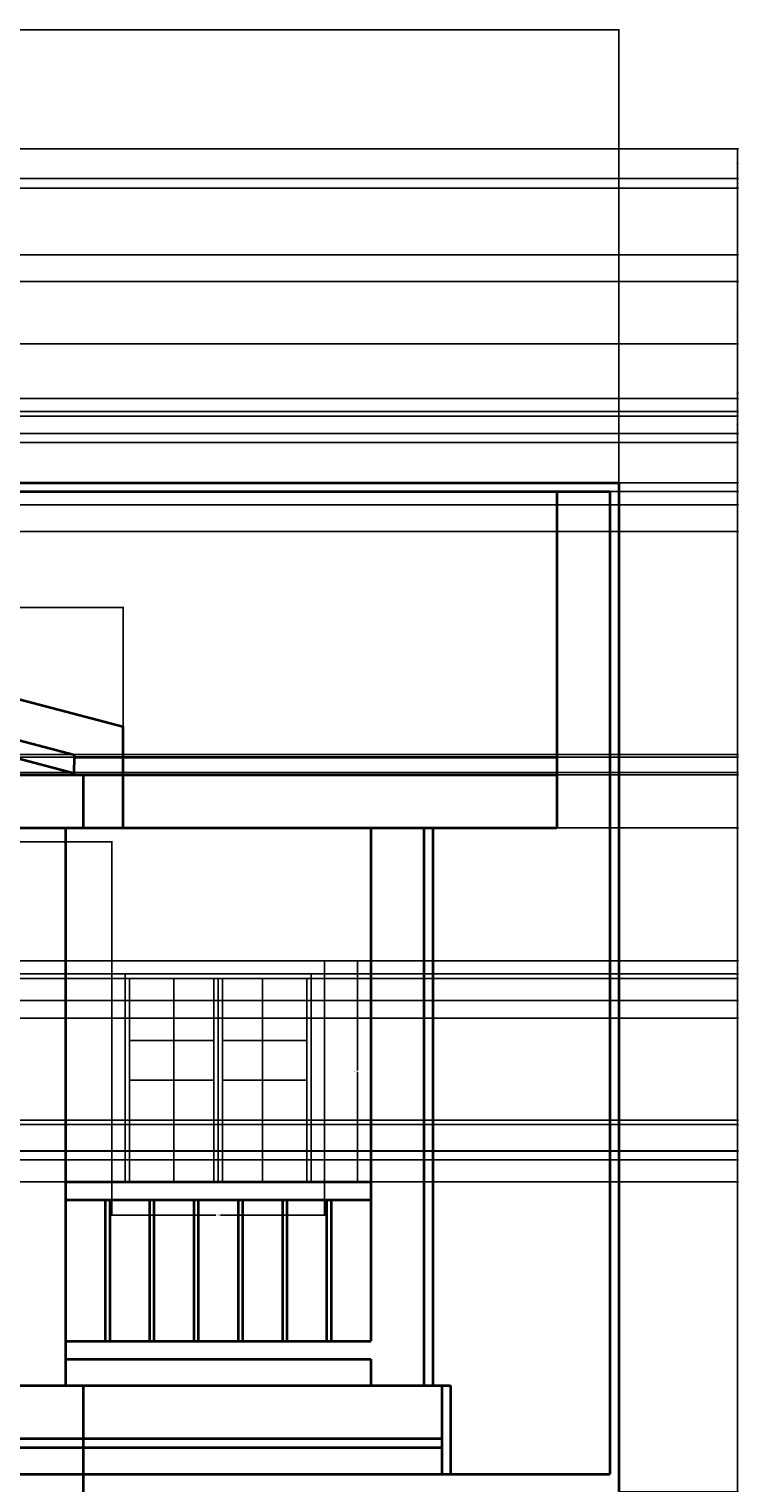
# Model space of a CAD drawing. Units: inches. Extents: x 2154 to 2740, y 571 to 1084.
# Tile 13 of 13: x 2580 to 2740, y 756 to 1084. Entities that reach past the tile are written whole.
import ezdxf

# ---------------------------------------------------------------- set-up
doc = ezdxf.new("R2010")
doc.units = ezdxf.units.IN
for name, color, linetype, lineweight in [('A-ANNO-DIMS', 2, 'Continuous', 18), ('A-ELEV', 7, 'Continuous', 35), ('A-GLAZ', 4, 'Continuous', 25), ('A-ROOF', 1, 'Continuous', 35)]:
    doc.layers.add(name, color=color, linetype=linetype, lineweight=lineweight)
doc.styles.get("Standard").update_dxf_attribs({"font": 'arial.ttf'})
doc.dimstyles.get("Standard").update_dxf_attribs({"dimtxt": 0.18, "dimasz": 0.18, "dimexe": 0.18, "dimexo": 0.0625, "dimgap": 0.09, "dimtad": 0, "dimtih": 1, "dimtoh": 1, "dimdec": 4, "dimzin": 0, "dimdsep": 46, "dimtxsty": 'Standard', "dimcen": 0.09, "dimadec": 0, "dimazin": 0, "dimtfac": 1, "dimtdec": 4, "dimtofl": 0, "dimtmove": 0, "dimatfit": 3, "dimfxl": 1, "dimtolj": 1, "dimtzin": 0, "dimarcsym": 0})

# ---------------------------------------------------------------- blocks, each defined once
blk = doc.blocks.new('WIN-ELEV-1200')
for p, q in [((0, 50), (48, 50)), ((0, 0), (0, 50)), ((48, 0), (48, 50)), ((3, 0), (3, 47)), ((3, 47), (45, 47)), ((4, 46), (44, 46)), ((4, 0), (4, 46)), ((14, 0), (14, 46)), ((23, 0), (23, 46)), ((24, 0), (24, 46)), ((25, 0), (25, 46)), ((34, 0), (34, 46)), ((44, 0), (44, 46)), ((45, 0), (45, 47)), ((4, 41), (23, 41)), ((25, 41), (44, 41)), ((4, 32), (23, 32)), ((25, 32), (44, 32)), ((4, 23), (23, 23)), ((25, 23), (44, 23)), ((4, 14), (23, 14)), ((25, 14), (44, 14)), ((4, 5), (23, 5)), ((25, 5), (44, 5))]:
    blk.add_line(p, q)
blk = doc.blocks.new('*D3')
at = {"layer": 'A-ANNO-DIMS', "color": 0, "lineweight": -2, "transparency": 16777216}
for p, q in [((2646.77, 873.53), (2654.39, 873.53)), ((2654.21, 873.35), (2654.21, 848.72)), ((2654.21, 823.71), (2654.21, 848.35)), ((2646.77, 823.53), (2654.39, 823.53))]:
    blk.add_line(p, q, dxfattribs=at)
at = {"layer": 'A-ANNO-DIMS', "color": 0, "transparency": 16777216}
for points in [[(2654.18, 873.35), (2654.24, 873.35), (2654.21, 873.53)], [(2654.18, 823.71), (2654.24, 823.71), (2654.21, 823.53)]]:
    blk.add_solid(points, dxfattribs=at)
at = {"layer": 'Defpoints', "color": 0, "transparency": 16777216}
for p in [(2646.71, 873.53), (2654.21, 873.53), (2646.71, 823.53)]:
    blk.add_point(p, dxfattribs=at)
at = {"layer": 'A-ANNO-DIMS', "color": 0, "transparency": 16777216, "insert": (2654.21, 848.53), "char_height": 0.18, "attachment_point": 5}
blk.add_mtext('\\A1;WINDOW 50 TYP.', dxfattribs=at)
blk = doc.blocks.new('*D4')
at = {"layer": 'A-ANNO-DIMS', "color": 0, "lineweight": -2, "transparency": 16777216}
for p, q in [((2598.71, 823.47), (2598.71, 815.85)), ((2646.71, 823.47), (2646.71, 815.85)), ((2598.89, 816.03), (2622.17, 816.03)), ((2646.53, 816.03), (2623.24, 816.03))]:
    blk.add_line(p, q, dxfattribs=at)
at = {"layer": 'A-ANNO-DIMS', "color": 0, "transparency": 16777216}
for points in [[(2598.89, 816.06), (2598.89, 816), (2598.71, 816.03)], [(2646.53, 816.06), (2646.53, 816), (2646.71, 816.03)]]:
    blk.add_solid(points, dxfattribs=at)
at = {"layer": 'Defpoints', "color": 0, "transparency": 16777216}
for p in [(2598.71, 823.53), (2646.71, 823.53), (2646.71, 816.03)]:
    blk.add_point(p, dxfattribs=at)
at = {"layer": 'A-ANNO-DIMS', "color": 0, "transparency": 16777216, "insert": (2622.71, 816.03), "char_height": 0.18, "attachment_point": 5}
blk.add_mtext('\\A1;48 TYP.', dxfattribs=at)
blk = doc.blocks.new('*D7')
at = {"layer": 'A-ANNO-DIMS', "color": 0, "lineweight": -2, "transparency": 16777216}
for p, q in [((2181.21, 981.59), (2181.21, 1084.04)), ((2181.39, 1083.86), (2446.92, 1083.86)), ((2713.03, 1083.86), (2447.49, 1083.86)), ((2713.21, 981.59), (2713.21, 1084.04))]:
    blk.add_line(p, q, dxfattribs=at)
at = {"layer": 'A-ANNO-DIMS', "color": 0, "transparency": 16777216}
for points in [[(2181.39, 1083.89), (2181.39, 1083.83), (2181.21, 1083.86)], [(2713.03, 1083.89), (2713.03, 1083.83), (2713.21, 1083.86)]]:
    blk.add_solid(points, dxfattribs=at)
at = {"layer": 'Defpoints', "color": 0, "transparency": 16777216}
for p in [(2713.21, 1083.86), (2181.21, 981.53), (2713.21, 981.53)]:
    blk.add_point(p, dxfattribs=at)
at = {"layer": 'A-ANNO-DIMS', "color": 0, "transparency": 16777216, "insert": (2447.21, 1083.86), "char_height": 0.18, "attachment_point": 5}
blk.add_mtext('\\A1;532', dxfattribs=at)
blk = doc.blocks.new('*D8')
at = {"layer": 'A-ANNO-DIMS', "color": 0, "lineweight": -2, "transparency": 16777216}
for p, q in [((2284.21, 926.63), (2284.21, 953.59)), ((2284.39, 953.41), (2442.43, 953.37)), ((2601.03, 953.33), (2443, 953.37)), ((2601.21, 926.54), (2601.21, 953.51))]:
    blk.add_line(p, q, dxfattribs=at)
at = {"layer": 'A-ANNO-DIMS', "color": 0, "transparency": 16777216}
for points in [[(2284.39, 953.44), (2284.39, 953.38), (2284.21, 953.41)], [(2601.03, 953.36), (2601.03, 953.3), (2601.21, 953.33)]]:
    blk.add_solid(points, dxfattribs=at)
at = {"layer": 'Defpoints', "color": 0, "transparency": 16777216}
for p in [(2601.21, 953.33), (2284.21, 926.56), (2601.21, 926.48)]:
    blk.add_point(p, dxfattribs=at)
at = {"layer": 'A-ANNO-DIMS', "color": 0, "transparency": 16777216, "insert": (2442.71, 953.37), "char_height": 0.18, "attachment_point": 5}
blk.add_mtext('\\A1;317', dxfattribs=at)
blk = doc.blocks.new('*D12')
at = {"layer": 'A-ANNO-DIMS', "color": 0, "lineweight": -2, "transparency": 16777216}
for p, q in [((2713.27, 981.53), (2740.24, 981.53)), ((2740.06, 981.35), (2740.06, 867.71)), ((2740.06, 753.71), (2740.06, 867.35)), ((2713.27, 753.53), (2740.24, 753.53))]:
    blk.add_line(p, q, dxfattribs=at)
at = {"layer": 'A-ANNO-DIMS', "color": 0, "transparency": 16777216}
for points in [[(2740.03, 981.35), (2740.09, 981.35), (2740.06, 981.53)], [(2740.03, 753.71), (2740.09, 753.71), (2740.06, 753.53)]]:
    blk.add_solid(points, dxfattribs=at)
at = {"layer": 'Defpoints', "color": 0, "transparency": 16777216}
for p in [(2713.21, 981.53), (2740.06, 981.53), (2713.21, 753.53)]:
    blk.add_point(p, dxfattribs=at)
at = {"layer": 'A-ANNO-DIMS', "color": 0, "transparency": 16777216, "insert": (2740.06, 867.53), "char_height": 0.18, "attachment_point": 5}
blk.add_mtext('\\A1;228', dxfattribs=at)
blk = doc.blocks.new('*D13')
at = {"layer": 'A-ANNO-DIMS', "color": 0, "lineweight": -2, "transparency": 16777216}
for p, q in [((2447.27, 1057.01), (2740.24, 1057.01)), ((2740.06, 1056.83), (2740.06, 1019.45)), ((2740.06, 981.71), (2740.06, 1019.09)), ((2713.27, 981.53), (2740.24, 981.53))]:
    blk.add_line(p, q, dxfattribs=at)
at = {"layer": 'A-ANNO-DIMS', "color": 0, "transparency": 16777216}
for points in [[(2740.03, 1056.83), (2740.09, 1056.83), (2740.06, 1057.01)], [(2740.03, 981.71), (2740.09, 981.71), (2740.06, 981.53)]]:
    blk.add_solid(points, dxfattribs=at)
at = {"layer": 'Defpoints', "color": 0, "transparency": 16777216}
for p in [(2447.21, 1057.01), (2740.06, 1057.01), (2713.21, 981.53)]:
    blk.add_point(p, dxfattribs=at)
at = {"layer": 'A-ANNO-DIMS', "color": 0, "transparency": 16777216, "insert": (2740.06, 1019.27), "char_height": 0.18, "attachment_point": 5}
blk.add_mtext('\\A1;75.47', dxfattribs=at)
blk = doc.blocks.new('*D30')
at = {"layer": 'A-ANNO-DIMS', "color": 0, "lineweight": -2, "transparency": 16777216}
for p, q in [((2657.14, 823.53), (2154.18, 823.53)), ((2154.36, 823.35), (2154.36, 800.71)), ((2154.36, 777.71), (2154.36, 800.35)), ((2657.14, 777.53), (2154.18, 777.53))]:
    blk.add_line(p, q, dxfattribs=at)
at = {"layer": 'A-ANNO-DIMS', "color": 0, "transparency": 16777216}
for points in [[(2154.33, 823.35), (2154.39, 823.35), (2154.36, 823.53)], [(2154.33, 777.71), (2154.39, 777.71), (2154.36, 777.53)]]:
    blk.add_solid(points, dxfattribs=at)
at = {"layer": 'Defpoints', "color": 0, "transparency": 16777216}
for p in [(2154.36, 823.53), (2657.21, 823.53), (2657.21, 777.53)]:
    blk.add_point(p, dxfattribs=at)
at = {"layer": 'A-ANNO-DIMS', "color": 0, "transparency": 16777216, "insert": (2154.36, 800.53), "char_height": 0.18, "attachment_point": 5}
blk.add_mtext('\\A1;46', dxfattribs=at)
blk = doc.blocks.new('*D42')
at = {"layer": 'A-ANNO-DIMS', "color": 0, "lineweight": -2, "transparency": 16777216}
for p, q in [((2517.68, 873.59), (2517.68, 900.56)), ((2517.86, 900.38), (2557.8, 900.38)), ((2598.53, 900.38), (2558.59, 900.38)), ((2598.71, 873.59), (2598.71, 900.56))]:
    blk.add_line(p, q, dxfattribs=at)
at = {"layer": 'A-ANNO-DIMS', "color": 0, "transparency": 16777216}
for points in [[(2517.86, 900.41), (2517.86, 900.35), (2517.68, 900.38)], [(2598.53, 900.41), (2598.53, 900.35), (2598.71, 900.38)]]:
    blk.add_solid(points, dxfattribs=at)
at = {"layer": 'Defpoints', "color": 0, "transparency": 16777216}
for p in [(2598.71, 900.38), (2517.68, 873.53), (2598.71, 873.53)]:
    blk.add_point(p, dxfattribs=at)
at = {"layer": 'A-ANNO-DIMS', "color": 0, "transparency": 16777216, "insert": (2558.19, 900.38), "char_height": 0.18, "attachment_point": 5}
blk.add_mtext('\\A1;81.03', dxfattribs=at)
blk = doc.blocks.new('*D46')
at = {"layer": 'A-ANNO-DIMS', "color": 0, "lineweight": -2, "transparency": 16777216}
for p, q in [((2195.27, 915.53), (2740.24, 915.53)), ((2740.06, 915.35), (2740.06, 909.71)), ((2740.06, 903.71), (2740.06, 909.35)), ((2195.27, 903.53), (2740.24, 903.53))]:
    blk.add_line(p, q, dxfattribs=at)
at = {"layer": 'A-ANNO-DIMS', "color": 0, "transparency": 16777216}
for points in [[(2740.03, 915.35), (2740.09, 915.35), (2740.06, 915.53)], [(2740.03, 903.71), (2740.09, 903.71), (2740.06, 903.53)]]:
    blk.add_solid(points, dxfattribs=at)
at = {"layer": 'Defpoints', "color": 0, "transparency": 16777216}
for p in [(2195.21, 915.53), (2740.06, 915.53), (2195.21, 903.53)]:
    blk.add_point(p, dxfattribs=at)
at = {"layer": 'A-ANNO-DIMS', "color": 0, "transparency": 16777216, "insert": (2740.06, 909.53), "char_height": 0.18, "attachment_point": 5}
blk.add_mtext('\\A1;12', dxfattribs=at)
blk = doc.blocks.new('*D47')
at = {"layer": 'A-ANNO-DIMS', "color": 0, "lineweight": -2, "transparency": 16777216}
for p, q in [((2195.269199, 919.532069), (2740.236699, 919.532069)), ((2740.056699, 919.352069), (2740.056699, 917.712069)), ((2740.056699, 915.712069), (2740.056699, 917.352069)), ((2195.269199, 915.532069), (2740.236699, 915.532069))]:
    blk.add_line(p, q, dxfattribs=at)
at = {"layer": 'A-ANNO-DIMS', "color": 0, "transparency": 16777216}
for points in [[(2740.026699, 919.352069), (2740.086699, 919.352069), (2740.056699, 919.532069)], [(2740.026699, 915.712069), (2740.086699, 915.712069), (2740.056699, 915.532069)]]:
    blk.add_solid(points, dxfattribs=at)
at = {"layer": 'Defpoints', "color": 0, "transparency": 16777216}
for p in [(2195.206699, 919.532069), (2740.056699, 919.532069), (2195.206699, 915.532069)]:
    blk.add_point(p, dxfattribs=at)
at = {"layer": 'A-ANNO-DIMS', "color": 0, "transparency": 16777216, "insert": (2740.056699, 917.532069), "char_height": 0.18, "attachment_point": 5}
blk.add_mtext('\\A1;4', dxfattribs=at)
blk = doc.blocks.new('*D48')
at = {"layer": 'A-ANNO-DIMS', "color": 0, "lineweight": -2, "transparency": 16777216}
for p, q in [((2195.27, 979.53), (2740.24, 979.53)), ((2740.06, 979.35), (2740.06, 949.71)), ((2740.06, 919.71), (2740.06, 949.35)), ((2195.27, 919.53), (2740.24, 919.53))]:
    blk.add_line(p, q, dxfattribs=at)
at = {"layer": 'A-ANNO-DIMS', "color": 0, "transparency": 16777216}
for points in [[(2740.03, 979.35), (2740.09, 979.35), (2740.06, 979.53)], [(2740.03, 919.71), (2740.09, 919.71), (2740.06, 919.53)]]:
    blk.add_solid(points, dxfattribs=at)
at = {"layer": 'Defpoints', "color": 0, "transparency": 16777216}
for p in [(2195.21, 979.53), (2740.06, 979.53), (2195.21, 919.53)]:
    blk.add_point(p, dxfattribs=at)
at = {"layer": 'A-ANNO-DIMS', "color": 0, "transparency": 16777216, "insert": (2740.06, 949.53), "char_height": 0.18, "attachment_point": 5}
blk.add_mtext('\\A1;60', dxfattribs=at)
blk = doc.blocks.new('*D55')
at = {"layer": 'A-ANNO-DIMS', "color": 0, "lineweight": -2, "transparency": 16777216}
for p, q in [((2295.84, 920.15), (2740.24, 920.15)), ((2740.06, 919.97), (2740.06, 918.27)), ((2740.06, 916.21), (2740.06, 917.91)), ((2295.83, 916.03), (2740.24, 916.03))]:
    blk.add_line(p, q, dxfattribs=at)
at = {"layer": 'A-ANNO-DIMS', "color": 0, "transparency": 16777216}
for points in [[(2740.03, 919.97), (2740.09, 919.97), (2740.06, 920.15)], [(2740.03, 916.21), (2740.09, 916.21), (2740.06, 916.03)]]:
    blk.add_solid(points, dxfattribs=at)
at = {"layer": 'Defpoints', "color": 0, "transparency": 16777216}
for p in [(2295.77, 920.15), (2740.06, 920.15), (2295.77, 916.03)]:
    blk.add_point(p, dxfattribs=at)
at = {"layer": 'A-ANNO-DIMS', "color": 0, "transparency": 16777216, "insert": (2740.06, 918.09), "char_height": 0.18, "attachment_point": 5}
blk.add_mtext('\\A1;4.12', dxfattribs=at)
blk = doc.blocks.new('*D69')
at = {"layer": 'A-ANNO-DIMS', "color": 0, "lineweight": -2, "transparency": 16777216}
for p, q in [((2447.27, 1057.01), (2740.24, 1057.01)), ((2740.06, 1056.83), (2740.06, 1053.83)), ((2740.06, 1050.47), (2740.06, 1053.47)), ((2447.27, 1050.29), (2740.24, 1050.29))]:
    blk.add_line(p, q, dxfattribs=at)
at = {"layer": 'A-ANNO-DIMS', "color": 0, "transparency": 16777216}
for points in [[(2740.03, 1056.83), (2740.09, 1056.83), (2740.06, 1057.01)], [(2740.03, 1050.47), (2740.09, 1050.47), (2740.06, 1050.29)]]:
    blk.add_solid(points, dxfattribs=at)
at = {"layer": 'Defpoints', "color": 0, "transparency": 16777216}
for p in [(2447.21, 1057.01), (2740.06, 1057.01), (2447.21, 1050.29)]:
    blk.add_point(p, dxfattribs=at)
at = {"layer": 'A-ANNO-DIMS', "color": 0, "transparency": 16777216, "insert": (2740.06, 1053.65), "char_height": 0.18, "attachment_point": 5}
blk.add_mtext('\\A1;6.712', dxfattribs=at)
blk = doc.blocks.new('*D70')
at = {"layer": 'A-ANNO-DIMS', "color": 0, "lineweight": -2, "transparency": 16777216}
for p, q in [((2447.27, 1050.29), (2740.24, 1050.29)), ((2447.27, 1048.06), (2740.24, 1048.06)), ((2740.06, 1050.11), (2740.06, 1049.36)), ((2740.06, 1048.24), (2740.06, 1048.99))]:
    blk.add_line(p, q, dxfattribs=at)
at = {"layer": 'A-ANNO-DIMS', "color": 0, "transparency": 16777216}
for points in [[(2740.03, 1050.11), (2740.09, 1050.11), (2740.06, 1050.29)], [(2740.03, 1048.24), (2740.09, 1048.24), (2740.06, 1048.06)]]:
    blk.add_solid(points, dxfattribs=at)
at = {"layer": 'Defpoints', "color": 0, "transparency": 16777216}
for p in [(2447.21, 1050.29), (2447.21, 1048.06), (2740.06, 1050.29)]:
    blk.add_point(p, dxfattribs=at)
at = {"layer": 'A-ANNO-DIMS', "color": 0, "transparency": 16777216, "insert": (2740.06, 1049.17), "char_height": 0.18, "attachment_point": 5}
blk.add_mtext('\\A1;2.24', dxfattribs=at)
blk = doc.blocks.new('*D71')
at = {"layer": 'A-ANNO-DIMS', "color": 0, "lineweight": -2, "transparency": 16777216}
for p, q in [((2477.27, 1033.01), (2740.24, 1033.01)), ((2740.06, 1032.83), (2740.06, 1030.2)), ((2740.06, 1027.19), (2740.06, 1029.83)), ((2477.27, 1027.01), (2740.24, 1027.01))]:
    blk.add_line(p, q, dxfattribs=at)
at = {"layer": 'A-ANNO-DIMS', "color": 0, "transparency": 16777216}
for points in [[(2740.03, 1032.83), (2740.09, 1032.83), (2740.06, 1033.01)], [(2740.03, 1027.19), (2740.09, 1027.19), (2740.06, 1027.01)]]:
    blk.add_solid(points, dxfattribs=at)
at = {"layer": 'Defpoints', "color": 0, "transparency": 16777216}
for p in [(2477.21, 1033.01), (2740.06, 1033.01), (2477.21, 1027.01)]:
    blk.add_point(p, dxfattribs=at)
at = {"layer": 'A-ANNO-DIMS', "color": 0, "transparency": 16777216, "insert": (2740.06, 1030.01), "char_height": 0.18, "attachment_point": 5}
blk.add_mtext('\\A1;6', dxfattribs=at)
blk = doc.blocks.new('*D72')
at = {"layer": 'A-ANNO-DIMS', "color": 0, "lineweight": -2, "transparency": 16777216}
for p, q in [((2477.27, 1027.01), (2740.24, 1027.01)), ((2740.06, 1026.83), (2740.06, 1001.96)), ((2740.06, 976.71), (2740.06, 1001.59)), ((2477.27, 976.53), (2740.24, 976.53))]:
    blk.add_line(p, q, dxfattribs=at)
at = {"layer": 'A-ANNO-DIMS', "color": 0, "transparency": 16777216}
for points in [[(2740.03, 1026.83), (2740.09, 1026.83), (2740.06, 1027.01)], [(2740.03, 976.71), (2740.09, 976.71), (2740.06, 976.53)]]:
    blk.add_solid(points, dxfattribs=at)
at = {"layer": 'Defpoints', "color": 0, "transparency": 16777216}
for p in [(2477.21, 1027.01), (2740.06, 1027.01), (2477.21, 976.53)]:
    blk.add_point(p, dxfattribs=at)
at = {"layer": 'A-ANNO-DIMS', "color": 0, "transparency": 16777216, "insert": (2740.06, 1001.77), "char_height": 0.18, "attachment_point": 5}
blk.add_mtext('\\A1;50.48', dxfattribs=at)
blk = doc.blocks.new('*D73')
at = {"layer": 'A-ANNO-DIMS', "color": 0, "lineweight": -2, "transparency": 16777216}
for p, q in [((2477.27, 976.53), (2740.24, 976.53)), ((2740.06, 976.35), (2740.06, 973.71)), ((2740.06, 970.71), (2740.06, 973.35)), ((2477.27, 970.53), (2740.24, 970.53))]:
    blk.add_line(p, q, dxfattribs=at)
at = {"layer": 'A-ANNO-DIMS', "color": 0, "transparency": 16777216}
for points in [[(2740.03, 976.35), (2740.09, 976.35), (2740.06, 976.53)], [(2740.03, 970.71), (2740.09, 970.71), (2740.06, 970.53)]]:
    blk.add_solid(points, dxfattribs=at)
at = {"layer": 'Defpoints', "color": 0, "transparency": 16777216}
for p in [(2477.21, 976.53), (2740.06, 976.53), (2477.21, 970.53)]:
    blk.add_point(p, dxfattribs=at)
at = {"layer": 'A-ANNO-DIMS', "color": 0, "transparency": 16777216, "insert": (2740.06, 973.53), "char_height": 0.18, "attachment_point": 5}
blk.add_mtext('\\A1;6', dxfattribs=at)
blk = doc.blocks.new('*D78')
at = {"layer": 'A-ANNO-DIMS', "color": 0, "lineweight": -2, "transparency": 16777216}
for p, q in [((2459.95, 1012.91), (2740.24, 1012.91)), ((2740.06, 1012.73), (2740.06, 1001.95)), ((2740.06, 990.82), (2740.06, 1001.59)), ((2459.95, 990.64), (2740.24, 990.64))]:
    blk.add_line(p, q, dxfattribs=at)
at = {"layer": 'A-ANNO-DIMS', "color": 0, "transparency": 16777216}
for points in [[(2740.03, 1012.73), (2740.09, 1012.73), (2740.06, 1012.91)], [(2740.03, 990.82), (2740.09, 990.82), (2740.06, 990.64)]]:
    blk.add_solid(points, dxfattribs=at)
at = {"layer": 'Defpoints', "color": 0, "transparency": 16777216}
for p in [(2459.89, 1012.91), (2740.06, 1012.91), (2459.89, 990.64)]:
    blk.add_point(p, dxfattribs=at)
at = {"layer": 'A-ANNO-DIMS', "color": 0, "transparency": 16777216, "insert": (2740.06, 1001.77), "char_height": 0.18, "attachment_point": 5}
blk.add_mtext('\\A1;22.27', dxfattribs=at)
blk = doc.blocks.new('*D83')
at = {"layer": 'A-ANNO-DIMS', "color": 0, "lineweight": -2, "transparency": 16777216}
for p, q in [((2457.95, 996.6), (2740.24, 996.6)), ((2740.06, 996.42), (2740.06, 994.8)), ((2457.95, 992.64), (2740.24, 992.64)), ((2740.06, 992.82), (2740.06, 994.44))]:
    blk.add_line(p, q, dxfattribs=at)
at = {"layer": 'A-ANNO-DIMS', "color": 0, "transparency": 16777216}
for points in [[(2740.03, 996.42), (2740.09, 996.42), (2740.06, 996.6)], [(2740.03, 992.82), (2740.09, 992.82), (2740.06, 992.64)]]:
    blk.add_solid(points, dxfattribs=at)
at = {"layer": 'Defpoints', "color": 0, "transparency": 16777216}
for p in [(2457.89, 996.6), (2740.06, 996.6), (2457.89, 992.64)]:
    blk.add_point(p, dxfattribs=at)
at = {"layer": 'A-ANNO-DIMS', "color": 0, "transparency": 16777216, "insert": (2740.06, 994.62), "char_height": 0.18, "attachment_point": 5}
blk.add_mtext('\\A1;3.964', dxfattribs=at)
blk = doc.blocks.new('*D84')
at = {"layer": 'A-ANNO-DIMS', "color": 0, "lineweight": -2, "transparency": 16777216}
for p, q in [((2457.95, 997.6), (2740.24, 997.6)), ((2457.95, 996.6), (2740.24, 996.6)), ((2740.06, 997.42), (2740.06, 997.28)), ((2740.06, 996.78), (2740.06, 996.92))]:
    blk.add_line(p, q, dxfattribs=at)
at = {"layer": 'A-ANNO-DIMS', "color": 0, "transparency": 16777216}
for points in [[(2740.03, 997.42), (2740.09, 997.42), (2740.06, 997.6)], [(2740.03, 996.78), (2740.09, 996.78), (2740.06, 996.6)]]:
    blk.add_solid(points, dxfattribs=at)
at = {"layer": 'Defpoints', "color": 0, "transparency": 16777216}
for p in [(2457.89, 997.6), (2457.89, 996.6), (2740.06, 997.6)]:
    blk.add_point(p, dxfattribs=at)
at = {"layer": 'A-ANNO-DIMS', "color": 0, "transparency": 16777216, "insert": (2740.06, 997.1), "char_height": 0.18, "attachment_point": 5}
blk.add_mtext('\\A1;1', dxfattribs=at)
blk = doc.blocks.new('*D85')
at = {"layer": 'A-ANNO-DIMS', "color": 0, "lineweight": -2, "transparency": 16777216}
for p, q in [((2457.95, 1000.6), (2740.24, 1000.6)), ((2740.06, 1000.42), (2740.06, 999.28)), ((2740.06, 997.78), (2740.06, 998.92)), ((2457.95, 997.6), (2740.24, 997.6))]:
    blk.add_line(p, q, dxfattribs=at)
at = {"layer": 'A-ANNO-DIMS', "color": 0, "transparency": 16777216}
for points in [[(2740.03, 1000.42), (2740.09, 1000.42), (2740.06, 1000.6)], [(2740.03, 997.78), (2740.09, 997.78), (2740.06, 997.6)]]:
    blk.add_solid(points, dxfattribs=at)
at = {"layer": 'Defpoints', "color": 0, "transparency": 16777216}
for p in [(2457.89, 1000.6), (2740.06, 1000.6), (2457.89, 997.6)]:
    blk.add_point(p, dxfattribs=at)
at = {"layer": 'A-ANNO-DIMS', "color": 0, "transparency": 16777216, "insert": (2740.06, 999.1), "char_height": 0.18, "attachment_point": 5}
blk.add_mtext('\\A1;3', dxfattribs=at)
blk = doc.blocks.new('*D100')
at = {"layer": 'A-ANNO-DIMS', "color": 0, "lineweight": -2, "transparency": 16777216}
for p, q in [((2472.769199, 873.532069), (2740.236699, 873.532069)), ((2740.056699, 873.352069), (2740.056699, 871.712069)), ((2740.056699, 869.712069), (2740.056699, 871.352069)), ((2468.769199, 869.532069), (2740.236699, 869.532069))]:
    blk.add_line(p, q, dxfattribs=at)
at = {"layer": 'A-ANNO-DIMS', "color": 0, "transparency": 16777216}
for points in [[(2740.026699, 873.352069), (2740.086699, 873.352069), (2740.056699, 873.532069)], [(2740.026699, 869.712069), (2740.086699, 869.712069), (2740.056699, 869.532069)]]:
    blk.add_solid(points, dxfattribs=at)
at = {"layer": 'Defpoints', "color": 0, "transparency": 16777216}
for p in [(2472.706699, 873.532069), (2468.706699, 869.532069), (2740.056699, 869.532069)]:
    blk.add_point(p, dxfattribs=at)
at = {"layer": 'A-ANNO-DIMS', "color": 0, "transparency": 16777216, "insert": (2740.056699, 871.532069), "char_height": 0.18, "attachment_point": 5}
blk.add_mtext('\\A1;4', dxfattribs=at)
blk = doc.blocks.new('*D106')
at = {"layer": 'A-ANNO-DIMS', "color": 0, "lineweight": -2, "transparency": 16777216}
for p, q in [((2459.769199, 830.532069), (2740.236699, 830.532069)), ((2740.056699, 830.352069), (2740.056699, 827.212069)), ((2740.056699, 823.712069), (2740.056699, 826.852069)), ((2459.769199, 823.532069), (2740.236699, 823.532069))]:
    blk.add_line(p, q, dxfattribs=at)
at = {"layer": 'A-ANNO-DIMS', "color": 0, "transparency": 16777216}
for points in [[(2740.026699, 830.352069), (2740.086699, 830.352069), (2740.056699, 830.532069)], [(2740.026699, 823.712069), (2740.086699, 823.712069), (2740.056699, 823.532069)]]:
    blk.add_solid(points, dxfattribs=at)
at = {"layer": 'Defpoints', "color": 0, "transparency": 16777216}
for p in [(2459.706699, 830.532069), (2740.056699, 830.532069), (2459.706699, 823.532069)]:
    blk.add_point(p, dxfattribs=at)
at = {"layer": 'A-ANNO-DIMS', "color": 0, "transparency": 16777216, "insert": (2740.056699, 827.032069), "char_height": 0.18, "attachment_point": 5}
blk.add_mtext('\\A1;7', dxfattribs=at)
blk = doc.blocks.new('*D107')
at = {"layer": 'A-ANNO-DIMS', "color": 0, "lineweight": -2, "transparency": 16777216}
for p, q in [((2459.77, 836.53), (2740.24, 836.53)), ((2740.06, 836.35), (2740.06, 833.71)), ((2740.06, 830.71), (2740.06, 833.35)), ((2459.77, 830.53), (2740.24, 830.53))]:
    blk.add_line(p, q, dxfattribs=at)
at = {"layer": 'A-ANNO-DIMS', "color": 0, "transparency": 16777216}
for points in [[(2740.03, 836.35), (2740.09, 836.35), (2740.06, 836.53)], [(2740.03, 830.71), (2740.09, 830.71), (2740.06, 830.53)]]:
    blk.add_solid(points, dxfattribs=at)
at = {"layer": 'Defpoints', "color": 0, "transparency": 16777216}
for p in [(2459.71, 836.53), (2740.06, 836.53), (2459.71, 830.53)]:
    blk.add_point(p, dxfattribs=at)
at = {"layer": 'A-ANNO-DIMS', "color": 0, "transparency": 16777216, "insert": (2740.06, 833.53), "char_height": 0.18, "attachment_point": 5}
blk.add_mtext('\\A1;6', dxfattribs=at)
blk = doc.blocks.new('*D108')
at = {"layer": 'A-ANNO-DIMS', "color": 0, "lineweight": -2, "transparency": 16777216}
for p, q in [((2459.77, 860.53), (2740.24, 860.53)), ((2740.06, 860.35), (2740.06, 848.71)), ((2740.06, 836.71), (2740.06, 848.35)), ((2459.77, 836.53), (2740.24, 836.53))]:
    blk.add_line(p, q, dxfattribs=at)
at = {"layer": 'A-ANNO-DIMS', "color": 0, "transparency": 16777216}
for points in [[(2740.03, 860.35), (2740.09, 860.35), (2740.06, 860.53)], [(2740.03, 836.71), (2740.09, 836.71), (2740.06, 836.53)]]:
    blk.add_solid(points, dxfattribs=at)
at = {"layer": 'Defpoints', "color": 0, "transparency": 16777216}
for p in [(2459.71, 860.53), (2740.06, 860.53), (2459.71, 836.53)]:
    blk.add_point(p, dxfattribs=at)
at = {"layer": 'A-ANNO-DIMS', "color": 0, "transparency": 16777216, "insert": (2740.06, 848.53), "char_height": 0.18, "attachment_point": 5}
blk.add_mtext('\\A1;24', dxfattribs=at)
blk = doc.blocks.new('*D109')
at = {"layer": 'A-ANNO-DIMS', "color": 0, "lineweight": -2, "transparency": 16777216}
for p, q in [((2468.77, 869.53), (2740.24, 869.53)), ((2740.06, 869.35), (2740.06, 865.21)), ((2740.06, 860.71), (2740.06, 864.85)), ((2459.77, 860.53), (2740.24, 860.53))]:
    blk.add_line(p, q, dxfattribs=at)
at = {"layer": 'A-ANNO-DIMS', "color": 0, "transparency": 16777216}
for points in [[(2740.03, 869.35), (2740.09, 869.35), (2740.06, 869.53)], [(2740.03, 860.71), (2740.09, 860.71), (2740.06, 860.53)]]:
    blk.add_solid(points, dxfattribs=at)
at = {"layer": 'Defpoints', "color": 0, "transparency": 16777216}
for p in [(2468.71, 869.53), (2740.06, 869.53), (2459.71, 860.53)]:
    blk.add_point(p, dxfattribs=at)
at = {"layer": 'A-ANNO-DIMS', "color": 0, "transparency": 16777216, "insert": (2740.06, 865.03), "char_height": 0.18, "attachment_point": 5}
blk.add_mtext('\\A1;9', dxfattribs=at)
blk = doc.blocks.new('*D112')
at = {"layer": 'A-ANNO-DIMS', "color": 0, "lineweight": -2, "transparency": 16777216}
for p, q in [((2291.32, 873.53), (2740.24, 873.53)), ((2740.06, 873.35), (2740.06, 872.21)), ((2740.06, 870.71), (2740.06, 871.85)), ((2288.32, 870.53), (2740.24, 870.53))]:
    blk.add_line(p, q, dxfattribs=at)
at = {"layer": 'A-ANNO-DIMS', "color": 0, "transparency": 16777216}
for points in [[(2740.03, 873.35), (2740.09, 873.35), (2740.06, 873.53)], [(2740.03, 870.71), (2740.09, 870.71), (2740.06, 870.53)]]:
    blk.add_solid(points, dxfattribs=at)
at = {"layer": 'Defpoints', "color": 0, "transparency": 16777216}
for p in [(2291.26, 873.53), (2740.06, 873.53), (2288.26, 870.53)]:
    blk.add_point(p, dxfattribs=at)
at = {"layer": 'A-ANNO-DIMS', "color": 0, "transparency": 16777216, "insert": (2740.06, 872.03), "char_height": 0.18, "attachment_point": 5}
blk.add_mtext('\\A1;3', dxfattribs=at)
blk = doc.blocks.new('*D119')
at = {"layer": 'A-ANNO-DIMS', "color": 0, "lineweight": -2, "transparency": 16777216}
for p, q in [((2287.32, 828.53), (2740.24, 828.53)), ((2740.06, 828.35), (2740.06, 826.21)), ((2740.06, 823.71), (2740.06, 825.85)), ((2287.32, 823.53), (2740.24, 823.53))]:
    blk.add_line(p, q, dxfattribs=at)
at = {"layer": 'A-ANNO-DIMS', "color": 0, "transparency": 16777216}
for points in [[(2740.03, 828.35), (2740.09, 828.35), (2740.06, 828.53)], [(2740.03, 823.71), (2740.09, 823.71), (2740.06, 823.53)]]:
    blk.add_solid(points, dxfattribs=at)
at = {"layer": 'Defpoints', "color": 0, "transparency": 16777216}
for p in [(2287.26, 828.53), (2740.06, 828.53), (2287.26, 823.53)]:
    blk.add_point(p, dxfattribs=at)
at = {"layer": 'A-ANNO-DIMS', "color": 0, "transparency": 16777216, "insert": (2740.06, 826.03), "char_height": 0.18, "attachment_point": 5}
blk.add_mtext('\\A1;5', dxfattribs=at)
blk = doc.blocks.new('*D120')
at = {"layer": 'A-ANNO-DIMS', "color": 0, "lineweight": -2, "transparency": 16777216}
for p, q in [((2287.32, 837.53), (2740.24, 837.53)), ((2740.06, 837.35), (2740.06, 833.21)), ((2740.06, 828.71), (2740.06, 832.85)), ((2287.32, 828.53), (2740.24, 828.53))]:
    blk.add_line(p, q, dxfattribs=at)
at = {"layer": 'A-ANNO-DIMS', "color": 0, "transparency": 16777216}
for points in [[(2740.03, 837.35), (2740.09, 837.35), (2740.06, 837.53)], [(2740.03, 828.71), (2740.09, 828.71), (2740.06, 828.53)]]:
    blk.add_solid(points, dxfattribs=at)
at = {"layer": 'Defpoints', "color": 0, "transparency": 16777216}
for p in [(2287.26, 837.53), (2740.06, 837.53), (2287.26, 828.53)]:
    blk.add_point(p, dxfattribs=at)
at = {"layer": 'A-ANNO-DIMS', "color": 0, "transparency": 16777216, "insert": (2740.06, 833.03), "char_height": 0.18, "attachment_point": 5}
blk.add_mtext('\\A1;9', dxfattribs=at)
blk = doc.blocks.new('*D121')
at = {"layer": 'A-ANNO-DIMS', "color": 0, "lineweight": -2, "transparency": 16777216}
for p, q in [((2287.32, 869.53), (2740.24, 869.53)), ((2740.06, 869.35), (2740.06, 867.21)), ((2287.32, 864.53), (2740.24, 864.53)), ((2740.06, 864.71), (2740.06, 866.85))]:
    blk.add_line(p, q, dxfattribs=at)
at = {"layer": 'A-ANNO-DIMS', "color": 0, "transparency": 16777216}
for points in [[(2740.03, 869.35), (2740.09, 869.35), (2740.06, 869.53)], [(2740.03, 864.71), (2740.09, 864.71), (2740.06, 864.53)]]:
    blk.add_solid(points, dxfattribs=at)
at = {"layer": 'Defpoints', "color": 0, "transparency": 16777216}
for p in [(2287.26, 869.53), (2740.06, 869.53), (2287.26, 864.53)]:
    blk.add_point(p, dxfattribs=at)
at = {"layer": 'A-ANNO-DIMS', "color": 0, "transparency": 16777216, "insert": (2740.06, 867.03), "char_height": 0.18, "attachment_point": 5}
blk.add_mtext('\\A1;5', dxfattribs=at)

msp = doc.modelspace()

# ---------------------------------------------------------------- linework, layer by layer
at = {"layer": 'A-ELEV'}
for p, q in [((2711.2067, 979.5321), (2711.2067, 757.5321)), ((2713.2067, 981.5321), (2713.2067, 753.5321)), ((2588.2067, 903.5321), (2588.2067, 777.5321)), ((2657.2067, 903.5321), (2657.2067, 787.5321)), ((2669.2067, 903.5321), (2669.2067, 777.5321)), ((2671.2067, 903.5321), (2671.2067, 777.5321)), ((2588.2067, 823.5321), (2657.2067, 823.5321)), ((2588.2067, 819.5321), (2657.2067, 819.5321)), ((2588.2067, 819.5321), (2588.2067, 787.5321)), ((2597.2067, 819.5321), (2597.2067, 787.5321)), ((2598.2067, 819.5321), (2598.2067, 787.5321)), ((2607.2067, 819.5321), (2607.2067, 787.5321)), ((2608.2067, 819.5321), (2608.2067, 787.5321)), ((2617.2067, 819.5321), (2617.2067, 787.5321)), ((2618.2067, 819.5321), (2618.2067, 787.5321)), ((2627.2067, 819.5321), (2627.2067, 787.5321)), ((2628.2067, 819.5321), (2628.2067, 787.5321)), ((2637.2067, 819.5321), (2637.2067, 787.5321)), ((2638.2067, 819.5321), (2638.2067, 787.5321)), ((2647.2067, 819.5321), (2647.2067, 787.5321)), ((2648.2067, 819.5321), (2648.2067, 787.5321)), ((2657.2067, 819.5321), (2657.2067, 787.5321)), ((2588.2067, 787.5321), (2657.2067, 787.5321)), ((2588.2067, 783.5321), (2657.2067, 783.5321)), ((2657.2067, 783.5321), (2657.2067, 777.5321)), ((2219.2067, 777.5321), (2675.2067, 777.5321)), ((2592.2067, 777.5321), (2592.2067, 753.5321)), ((2673.2067, 777.5321), (2673.2067, 757.5321)), ((2675.2067, 777.5321), (2675.2067, 757.5321)), ((2221.2067, 765.5321), (2673.2067, 765.5321)), ((2221.2067, 763.5321), (2673.2067, 763.5321)), ((2183.2067, 757.5321), (2711.2067, 757.5321))]:
    msp.add_line(p, q, dxfattribs=at)
at = {"layer": 'A-ROOF'}
for p, q in [((2477.2067, 981.5321), (2713.2067, 981.5321)), ((2477.2067, 979.5321), (2711.2067, 979.5321)), ((2699.2067, 979.5321), (2699.2067, 903.5321)), ((2447.273, 966.8186), (2601.2067, 926.4774)), ((2447.2067, 957.5321), (2590.2325, 920.0494)), ((2447.1772, 953.4047), (2590.1732, 915.9299)), ((2601.2067, 926.4774), (2601.2067, 903.5321)), ((2590.1675, 915.5321), (2590.2325, 920.0494)), ((2590.2251, 919.5321), (2699.2067, 919.5321)), ((2195.2067, 915.5321), (2699.2067, 915.5321)), ((2592.2067, 915.5321), (2592.2067, 903.5321)), ((2195.2067, 903.5321), (2699.2067, 903.5321))]:
    msp.add_line(p, q, dxfattribs=at)

# ---------------------------------------------------------------- block references
at = {"layer": 'A-GLAZ'}
msp.add_blockref('WIN-ELEV-1200', (2598.707, 823.532), dxfattribs=at)

# ---------------------------------------------------------------- dimensions: what is measured, and where the dimension line sits
at = {"layer": 'A-ANNO-DIMS'}
for base, p1, p2, override, picture, middle in [((2713.2067, 1083.8553), (2181.2067, 981.5321), (2713.2067, 981.5321), {"dimdec": 0, "dimlfac": 1, "dimrnd": 0, "dimzin": 0, "dimdsep": 46, "dimlunit": 2}, '*D7', (2447.2067, 1083.8553)), ((2598.7067, 900.3821), (2517.6813, 873.5321), (2598.7067, 873.5321), {"dimdec": 2, "dimlfac": 1, "dimrnd": 0, "dimzin": 0, "dimdsep": 46, "dimlunit": 2}, '*D42', (2558.194, 900.3821))]:
    dim = msp.add_linear_dim(base=base, p1=p1, p2=p2, dimstyle='Standard', override=override, dxfattribs=at)
    dim.commit()
    dim.dimension.update_dxf_attribs({"geometry": picture, "text_midpoint": middle})
for base, p1, p2, angle, override, picture, middle in [((2740.0567, 1057.0053), (2713.2067, 981.5321), (2447.2067, 1057.0053), 90, {"dimdec": 2, "dimlfac": 1, "dimrnd": 0, "dimzin": 0, "dimdsep": 46, "dimlunit": 2}, '*D13', (2740.0567, 1019.2687)), ((2740.0567, 1057.0053), (2447.2067, 1050.2934), (2447.2067, 1057.0053), 90, {"dimdec": 3, "dimlfac": 1, "dimrnd": 0, "dimzin": 0, "dimdsep": 46, "dimlunit": 2}, '*D69', (2740.0567, 1053.6493)), ((2740.0567, 1050.2934), (2447.2067, 1048.0561), (2447.2067, 1050.2934), 90, {"dimdec": 2, "dimlfac": 1, "dimrnd": 0, "dimzin": 0, "dimdsep": 46, "dimlunit": 2}, '*D70', (2740.0567, 1049.1747)), ((2740.0567, 1033.0148), (2477.2067, 1027.0148), (2477.2067, 1033.0148), 90, {"dimdec": 0, "dimlfac": 1, "dimrnd": 0, "dimzin": 0, "dimdsep": 46, "dimlunit": 2}, '*D71', (2740.0567, 1030.0148)), ((2740.0567, 1027.0148), (2477.2067, 976.5321), (2477.2067, 1027.0148), 90, {"dimdec": 2, "dimlfac": 1, "dimrnd": 0, "dimzin": 0, "dimdsep": 46, "dimlunit": 2}, '*D72', (2740.0567, 1001.7734)), ((2740.0567, 1012.9076), (2459.8896, 990.6361), (2459.8896, 1012.9076), 90, {"dimdec": 2, "dimlfac": 1, "dimrnd": 0, "dimzin": 0, "dimdsep": 46, "dimlunit": 2}, '*D78', (2740.0567, 1001.7719)), ((2740.0567, 1000.5998), (2457.8896, 997.5998), (2457.8896, 1000.5998), 90, {"dimdec": 0, "dimlfac": 1, "dimrnd": 0, "dimzin": 0, "dimdsep": 46, "dimlunit": 2}, '*D85', (2740.0567, 999.0998)), ((2740.0567, 997.5998), (2457.8896, 996.5998), (2457.8896, 997.5998), 90, {"dimdec": 0, "dimlfac": 1, "dimrnd": 0, "dimzin": 0, "dimdsep": 46, "dimlunit": 2}, '*D84', (2740.0567, 997.0998)), ((2740.0567, 996.5998), (2457.8896, 992.6361), (2457.8896, 996.5998), 90, {"dimdec": 3, "dimlfac": 1, "dimrnd": 0, "dimzin": 0, "dimdsep": 46, "dimlunit": 2}, '*D83', (2740.0567, 994.618)), ((2740.0567, 979.5321), (2195.2067, 919.5321), (2195.2067, 979.5321), 90, {"dimdec": 0, "dimlfac": 1, "dimrnd": 0, "dimzin": 0, "dimdsep": 46, "dimlunit": 2}, '*D48', (2740.0567, 949.5321)), ((2740.0567, 981.5321), (2713.2067, 753.5321), (2713.2067, 981.5321), 90, {"dimdec": 0, "dimlfac": 1, "dimrnd": 0, "dimzin": 0, "dimdsep": 46, "dimlunit": 2}, '*D12', (2740.0567, 867.5321)), ((2740.0567, 976.5321), (2477.2067, 970.5321), (2477.2067, 976.5321), 90, {"dimdec": 0, "dimlfac": 1, "dimrnd": 0, "dimzin": 0, "dimdsep": 46, "dimlunit": 2}, '*D73', (2740.0567, 973.5321)), ((2601.214, 953.3274), (2284.2067, 926.5633), (2601.2067, 926.4774), 359.984471, {"dimdec": 0, "dimlfac": 1, "dimrnd": 0, "dimzin": 0, "dimdsep": 46, "dimlunit": 2}, '*D8', (2442.714, 953.3703)), ((2740.0567, 920.1485), (2295.7714, 916.028), (2295.7731, 920.1485), 90, {"dimdec": 2, "dimlfac": 1, "dimrnd": 0, "dimzin": 0, "dimdsep": 46, "dimlunit": 2}, '*D55', (2740.0567, 918.0882)), ((2740.0567, 919.5321), (2195.2067, 915.5321), (2195.2067, 919.5321), 90, {"dimdec": 0, "dimlfac": 1, "dimrnd": 0, "dimzin": 0, "dimdsep": 46, "dimlunit": 2}, '*D47', (2740.0567, 917.5321)), ((2740.0567, 915.5321), (2195.2067, 903.5321), (2195.2067, 915.5321), 90, {"dimdec": 0, "dimlfac": 1, "dimrnd": 0, "dimzin": 0, "dimdsep": 46, "dimlunit": 2}, '*D46', (2740.0567, 909.5321)), ((2740.0567, 873.5321), (2288.2568, 870.5321), (2291.2568, 873.5321), 90, {"dimdec": 0, "dimlfac": 1, "dimrnd": 0, "dimzin": 0, "dimdsep": 46, "dimlunit": 2}, '*D112', (2740.0567, 872.0321)), ((2740.0567, 869.5321), (2472.7067, 873.5321), (2468.7067, 869.5321), 90, {"dimdec": 0, "dimlfac": 1, "dimrnd": 0, "dimzin": 0, "dimdsep": 46, "dimlunit": 2}, '*D100', (2740.0567, 871.5321)), ((2740.0567, 869.5321), (2287.2568, 864.5321), (2287.2568, 869.5321), 90, {"dimdec": 0, "dimlfac": 1, "dimrnd": 0, "dimzin": 0, "dimdsep": 46, "dimlunit": 2}, '*D121', (2740.0567, 867.0321)), ((2740.0567, 869.5321), (2459.7067, 860.5321), (2468.7067, 869.5321), 90, {"dimdec": 0, "dimlfac": 1, "dimrnd": 0, "dimzin": 0, "dimdsep": 46, "dimlunit": 2}, '*D109', (2740.0567, 865.0321)), ((2740.0567, 860.5321), (2459.7067, 836.5321), (2459.7067, 860.5321), 90, {"dimdec": 0, "dimlfac": 1, "dimrnd": 0, "dimzin": 0, "dimdsep": 46, "dimlunit": 2}, '*D108', (2740.0567, 848.5321)), ((2740.0567, 837.5321), (2287.2568, 828.5321), (2287.2568, 837.5321), 90, {"dimdec": 0, "dimlfac": 1, "dimrnd": 0, "dimzin": 0, "dimdsep": 46, "dimlunit": 2}, '*D120', (2740.0567, 833.0321)), ((2740.0567, 836.5321), (2459.7067, 830.5321), (2459.7067, 836.5321), 90, {"dimdec": 0, "dimlfac": 1, "dimrnd": 0, "dimzin": 0, "dimdsep": 46, "dimlunit": 2}, '*D107', (2740.0567, 833.5321)), ((2740.0567, 828.5321), (2287.2568, 823.5321), (2287.2568, 828.5321), 90, {"dimdec": 0, "dimlfac": 1, "dimrnd": 0, "dimzin": 0, "dimdsep": 46, "dimlunit": 2}, '*D119', (2740.0567, 826.0321)), ((2740.0567, 830.5321), (2459.7067, 823.5321), (2459.7067, 830.5321), 90, {"dimdec": 0, "dimlfac": 1, "dimrnd": 0, "dimzin": 0, "dimdsep": 46, "dimlunit": 2}, '*D106', (2740.0567, 827.0321)), ((2154.3567, 823.5321), (2657.2067, 777.5321), (2657.2067, 823.5321), 90, {"dimdec": 0, "dimlfac": 1, "dimrnd": 0, "dimzin": 0, "dimdsep": 46, "dimlunit": 2}, '*D30', (2154.3567, 800.5321))]:
    dim = msp.add_linear_dim(base=base, p1=p1, p2=p2, angle=angle, dimstyle='Standard', override=override, dxfattribs=at)
    dim.commit()
    dim.dimension.update_dxf_attribs({"geometry": picture, "text_midpoint": middle})
dim = msp.add_linear_dim(base=(2654.2067, 873.5321), p1=(2646.7067, 823.5321), p2=(2646.7067, 873.5321), angle=90, text='WINDOW <> TYP.', dimstyle='Standard', override={"dimdec": 0, "dimlfac": 1, "dimrnd": 0, "dimzin": 0, "dimdsep": 46, "dimlunit": 2}, dxfattribs=at)
dim.commit()
dim.dimension.update_dxf_attribs({"geometry": '*D3', "text_midpoint": (2654.2067, 848.5321)})
dim = msp.add_linear_dim(base=(2646.7067, 816.0321), p1=(2598.7067, 823.5321), p2=(2646.7067, 823.5321), text='<> TYP.', dimstyle='Standard', override={"dimdec": 0, "dimlfac": 1, "dimrnd": 0, "dimzin": 0, "dimdsep": 46, "dimlunit": 2}, dxfattribs=at)
dim.commit()
dim.dimension.update_dxf_attribs({"geometry": '*D4', "text_midpoint": (2622.7067, 816.0321)})

doc.saveas('drawing.dxf')
